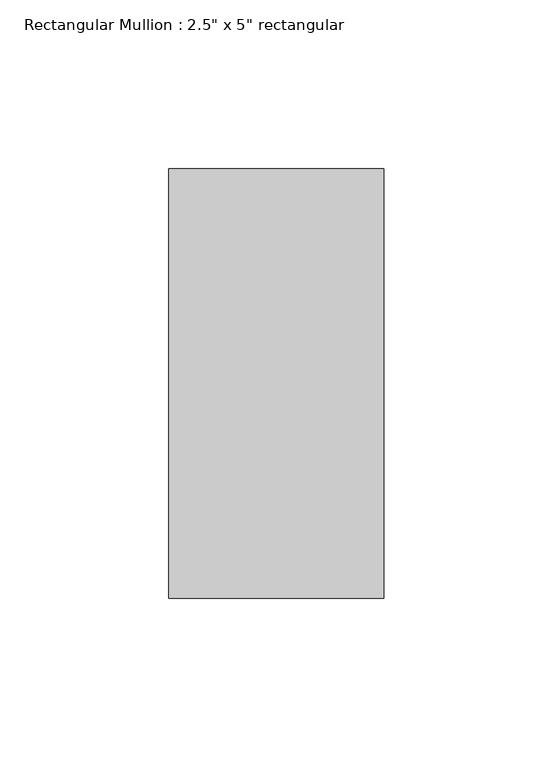
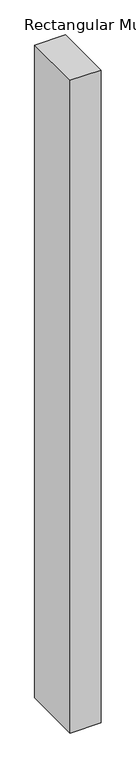
"""IFC4 building model written with IfcOpenShell, lengths in millimetres: member geometry."""

from ifc_helpers import new_model, si_unit, frame, origin, place, context, project, spatial, polyline, outline, extrude, source, transform, mapped, element, save


def member_6283365f(model_context):
    return source(origin(), model_context, "Body", "SweptSolid", [
        extrude(outline(polyline([(31.75, 63.5), (31.75, -63.5), (-31.75, -63.5), (-31.75, 63.5), (31.75, 63.5)])), frame((0.0, 0.0, -1422.1292854), z_axis=(0.0, 0.0, 1.0), x_axis=(1.0, 0.0, 0.0)), (0.0, 0.0, 1.0), 1422.1292854),
    ])


if __name__ == "__main__":
    model = new_model("IFC4")
    model_context = context("Model", 3, world=origin())
    ifc_project = project(units=[si_unit("LENGTHUNIT", "METRE", prefix="MILLI")], contexts=[model_context])
    site = spatial("IfcSite", under=ifc_project)
    building = spatial("IfcBuilding", under=site)
    placement = place(None, origin())
    member_shape = member_6283365f(model_context)
    element("IfcMember", 1, ObjectType="Rectangular Mullion : 2.5\" x 5\" rectangular", at=placement, inside=building, context=model_context, shape_type="MappedRepresentation", body=[
        mapped(member_shape, transform((0.0, 0.0, 0.0), x_axis=(1.0, 0.0, 0.0), y_axis=(0.0, 1.0, 0.0), z_axis=(0.0, 0.0, 1.0))),
    ])
    save(model, "model.ifc")

# Revit data of these elements
# Type "Rectangular Mullion : 2.5\" x 5\" rectangular"
#   built-in parameter 1007304 = 0.416667 (stored number, unit not read)
#   built-in parameter 1007301 = 0.104167 (stored number, unit not read)
#   built-in parameter 1007300 = 0.104167 (stored number, unit not read)
# Element 1 (IfcMember, "Rectangular Mullion : 2.5\" x 5\" rectangular")
#   Materials on its faces: "Aluminum"
# Materials
#   "Aluminum": class "Metal", colour RGB 247 247 247, transparency 0, Description = "Aluminum 6061", Cost = 0
